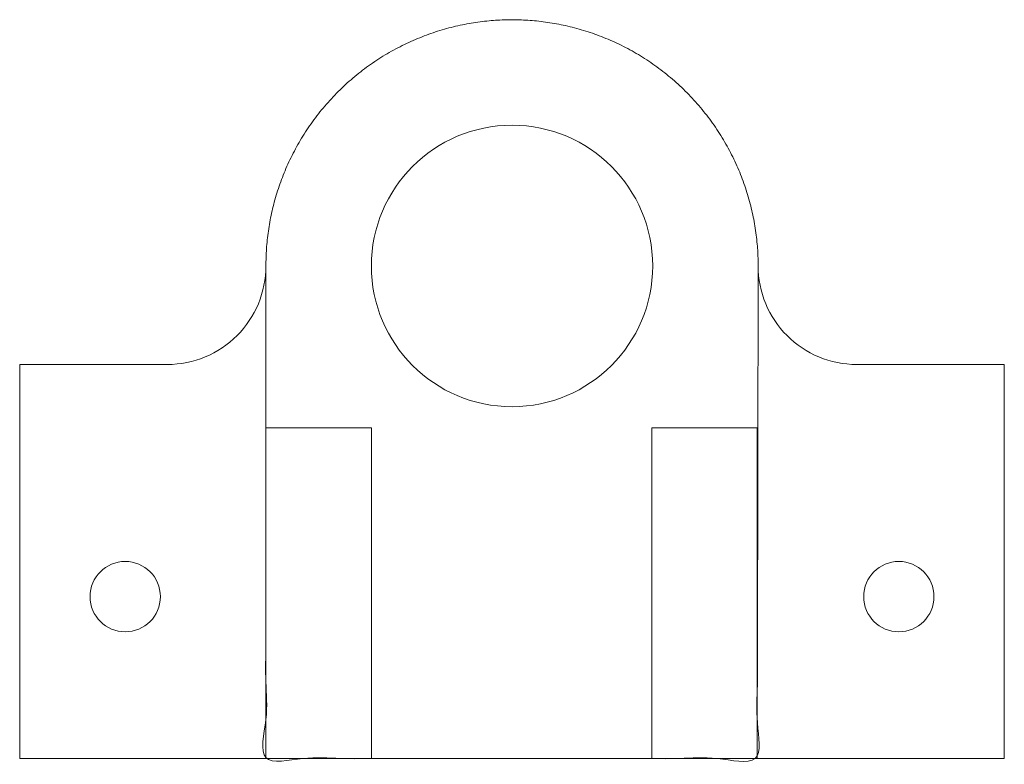
# Model space of a CAD drawing. Units: millimetres. Extents: x 2486 to 2626, y 1008 to 1114.
import ezdxf

# ---------------------------------------------------------------- set-up
doc = ezdxf.new("R2010")
doc.units = ezdxf.units.MM
doc.layers.add('M-CONS', color=8, linetype='Continuous', lineweight=18)

msp = doc.modelspace()

# ---------------------------------------------------------------- linework, layer by layer
at = {"layer": 'M-CONS'}
for p, q in [((2590.81, 1078.87), (2590.81, 1078.87)), ((2485.81, 1008.87), (2485.81, 1031.87)), ((2625.81, 1008.87), (2625.81, 1031.87))]:
    msp.add_line(p, q, dxfattribs=at)
at = {"layer": 'M-CONS', "extrusion": (0, -1, 0)}
msp.add_line((2590.81, 1078.87), (2590.81, 1078.87), dxfattribs=at)
at = {"layer": 'M-CONS', "extrusion": (-1, 0, 0)}
msp.add_line((2520.81, 1038.87, -65), (2520.81, 1055.87, -30), dxfattribs=at)
at = {"layer": 'M-CONS', "extrusion": (0, 0, -1)}
msp.add_line((2535.81, 1008.87), (2528.34, 1008.87), dxfattribs=at)
at = {"layer": 'M-CONS'}
msp.add_lwpolyline([(2590.81, 1078.87, 0.414214), (2604.81, 1064.87), (2625.81, 1064.87), (2625.81, 1008.87), (2485.81, 1008.87), (2485.81, 1064.87), (2506.81, 1064.87, 0.414214), (2520.81, 1078.87)], format="xyb", dxfattribs=at)
for points in [[(2535.81, 1055.87, 0), (2520.81, 1055.87, 0), (2520.81, 1008.87, 0), (2535.81, 1008.87, 0)], [(2590.69, 1055.87, 0), (2575.69, 1055.87, 0), (2575.69, 1008.87, 0), (2590.69, 1008.87, 0)]]:
    msp.add_polyline3d(points, close=True, dxfattribs=at)
for centre, radius in [((2555.81, 1078.87), 20), ((2500.81, 1031.87), 5), ((2610.81, 1031.87), 5)]:
    msp.add_circle(centre, radius, dxfattribs=at)
at = {"layer": 'M-CONS', "extrusion": (-1, 0, 0)}
msp.add_circle((-1023.87, -65, -2520.81), 5, dxfattribs=at)
at = {"layer": 'M-CONS', "extrusion": (1, 0, 0)}
msp.add_circle((1023.87, -65, 2575.69), 5, dxfattribs=at)
at = {"layer": 'M-CONS'}
msp.add_rational_spline([(2520.81, 1078.87), (2520.81, 1113.87), (2555.81, 1113.87), (2590.81, 1113.87), (2590.81, 1078.87), (2590.75, 1043.87), (2590.69, 1008.87), (2555.75, 1008.87), (2520.81, 1008.87), (2520.81, 1043.87), (2520.81, 1078.87)], [1, 0.707106781187, 1, 0.707106781187, 1, 1, 1, 1, 1, 1, 1], degree=2, knots=[0, 0, 0, 1.570796, 1.570796, 3.141593, 3.141593, 4.141593, 4.141593, 5.141593, 5.141593, 6.141593, 6.141593, 6.141593], dxfattribs=at)

doc.saveas('drawing.dxf')
